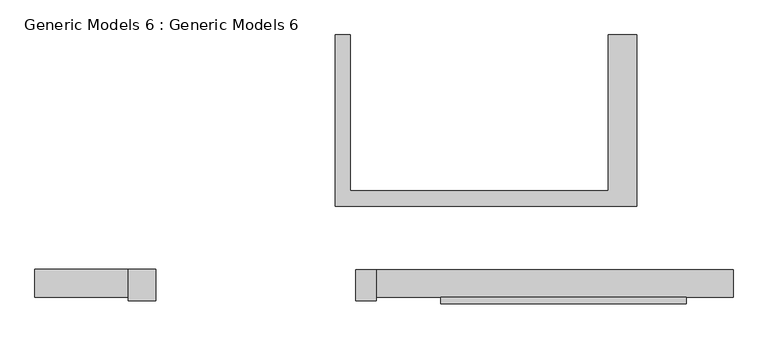
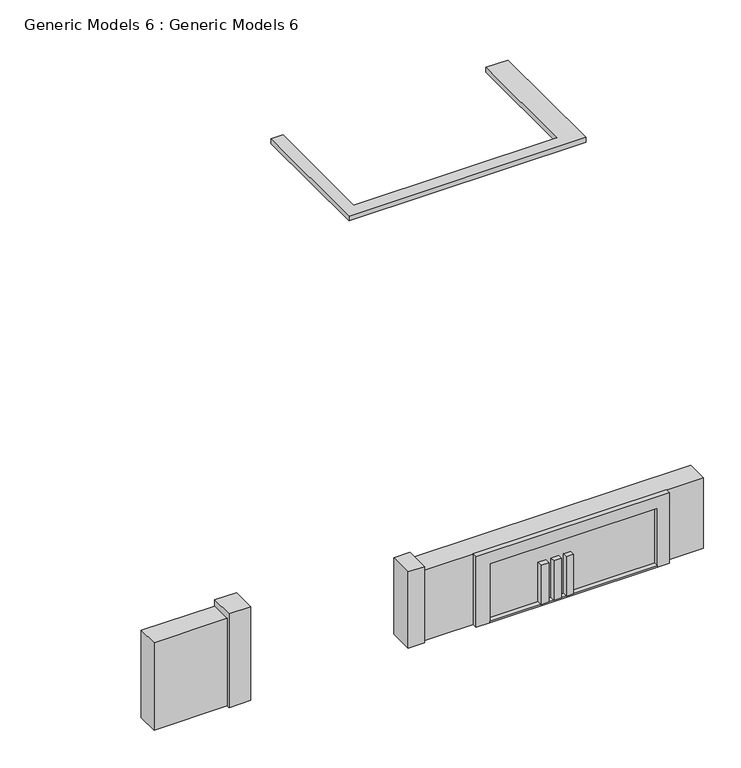
"""IFC4 building model written with IfcOpenShell, lengths in millimetres: proxy geometry, Generic Models 6 : Generic Models 6."""

from ifc_helpers import new_model, si_unit, frame, origin, place, context, project, spatial, polyline, outline, extrude, source, transform, mapped, element, save


def generic_models_6_generic_models_6_42a028d1(model_context):
    return source(origin(), model_context, "Body", "SweptSolid", [
        extrude(outline(polyline([(-8268.129521, -16830.0001929), (-8471.329521, -16830.0001929), (-8471.329521, -16703.0001929), (-8268.129521, -16703.0001929), (-8268.129521, -16830.0001929)])), frame((0.0, 0.0, -269.9597342), z_axis=(0.0, 0.0, 1.0), x_axis=(1.0, 0.0, 0.0)), (0.0, 0.0, 1.0), 1020.5382285),
        extrude(outline(polyline([(-7963.329521, -16830.0001929), (-8153.829521, -16830.0001929), (-8153.829521, -16703.0001929), (-7963.329521, -16703.0001929), (-7963.329521, -16830.0001929)])), frame((0.0, 0.0, -269.9597342), z_axis=(0.0, 0.0, 1.0), x_axis=(1.0, 0.0, 0.0)), (0.0, 0.0, 1.0), 1020.5382285),
        extrude(outline(polyline([(-7669.0219959, -16830.0001929), (-7842.679521, -16830.0001929), (-7842.679521, -16703.0001929), (-7669.0219959, -16703.0001929), (-7669.0219959, -16830.0001929)])), frame((0.0, 0.0, -269.9597342), z_axis=(0.0, 0.0, 1.0), x_axis=(1.0, 0.0, 0.0)), (0.0, 0.0, 1.0), 1020.5382285),
        extrude(outline(polyline([(-5601.129521, -16703.0001929), (-5601.129521, -16830.0001929), (-9715.929521, -16830.0001929), (-9715.929521, -16703.0001929), (-5601.129521, -16703.0001929)])), frame((0.0, 0.0, -304.8), z_axis=(0.0, 0.0, 1.0), x_axis=(1.0, 0.0, 0.0)), (0.0, 0.0, 1.0), 34.8402658),
        extrude(outline(polyline([(1525.1327889, -10061.2156184), (-304.8, -10061.2156184), (-304.8, -9715.929521), (1220.3327889, -9715.929521), (1220.3327889, -5601.129521), (-304.8, -5601.129521), (-304.8, -5311.72905), (1525.1327889, -5311.72905), (1525.1327889, -10061.2156184)])), frame((0.0, -16830.0001929, 0.0), z_axis=(0.0, 1.0, 0.0), x_axis=(0.0, 0.0, 1.0)), (0.0, 0.0, 1.0), 127.0),
        extrude(outline(polyline([(-15570.629521, -16169.6001929), (-15570.629521, -16776.4258181), (-16104.029521, -16776.4258181), (-16104.029521, -16169.6001929), (-15570.629521, -16169.6001929)])), frame((0.0, 0.0, -304.8), z_axis=(0.0, 0.0, 1.0), x_axis=(1.0, 0.0, 0.0)), (0.0, 0.0, 1.0), 2432.8057339),
        extrude(outline(polyline([(-11699.7085197, -16776.4258181), (-11699.7085197, -16169.6001929), (-11303.429521, -16169.6001929), (-11303.429521, -16776.4258181), (-11699.7085197, -16776.4258181)])), frame((0.0, 0.0, -304.8), z_axis=(0.0, 0.0, 1.0), x_axis=(1.0, 0.0, 0.0)), (0.0, 0.0, 1.0), 1981.1345144),
        extrude(outline(polyline([(-16104.029521, -16703.0001929), (-17905.1468092, -16703.0001929), (-17905.1468092, -16169.6001929), (-16104.029521, -16169.6001929), (-16104.029521, -16703.0001929)])), frame((0.0, 0.0, -304.8), z_axis=(0.0, 0.0, 1.0), x_axis=(1.0, 0.0, 0.0)), (0.0, 0.0, 1.0), 2268.8201935),
        extrude(outline(polyline([(-4407.329521, -16703.0001929), (-11303.429521, -16703.0001929), (-11303.429521, -16169.6001929), (-4407.329521, -16169.6001929), (-4407.329521, -16703.0001929)])), frame((0.0, 0.0, -304.8), z_axis=(0.0, 0.0, 1.0), x_axis=(1.0, 0.0, 0.0)), (0.0, 0.0, 1.0), 1829.9327889),
        extrude(outline(polyline([(-6274.229521, -14950.4001929), (-12103.529521, -14950.4001929), (-12103.529521, -11635.7001929), (-11810.7172113, -11635.7001929), (-11810.7172113, -14645.6001929), (-6816.9648193, -14645.6001929), (-6816.9648193, -11635.7001929), (-6274.229521, -11635.7001929), (-6274.229521, -14950.4001929)])), frame((0.0, 0.0, 9822.6068762), z_axis=(0.0, 0.0, 1.0), x_axis=(1.0, 0.0, 0.0)), (0.0, 0.0, 1.0), 127.0),
    ])


if __name__ == "__main__":
    model = new_model("IFC4")
    model_context = context("Model", 3, world=origin())
    ifc_project = project(units=[si_unit("LENGTHUNIT", "METRE", prefix="MILLI")], contexts=[model_context])
    site = spatial("IfcSite", under=ifc_project)
    building = spatial("IfcBuilding", under=site)
    placement = place(None, origin())
    generic_models_6_generic_models_6_shape = generic_models_6_generic_models_6_42a028d1(model_context)
    element("IfcBuildingElementProxy", 1, Name="Generic Models 6 : Generic Models 6", ObjectType="Generic Models 6 : Generic Models 6", at=placement, inside=building, context=model_context, shape_type="MappedRepresentation", body=[
        mapped(generic_models_6_generic_models_6_shape, transform((0.0, 0.0, 0.0), x_axis=(1.0, 0.0, 0.0), y_axis=(0.0, 1.0, 0.0), z_axis=(0.0, 0.0, 1.0))),
    ])
    save(model, "model.ifc")
